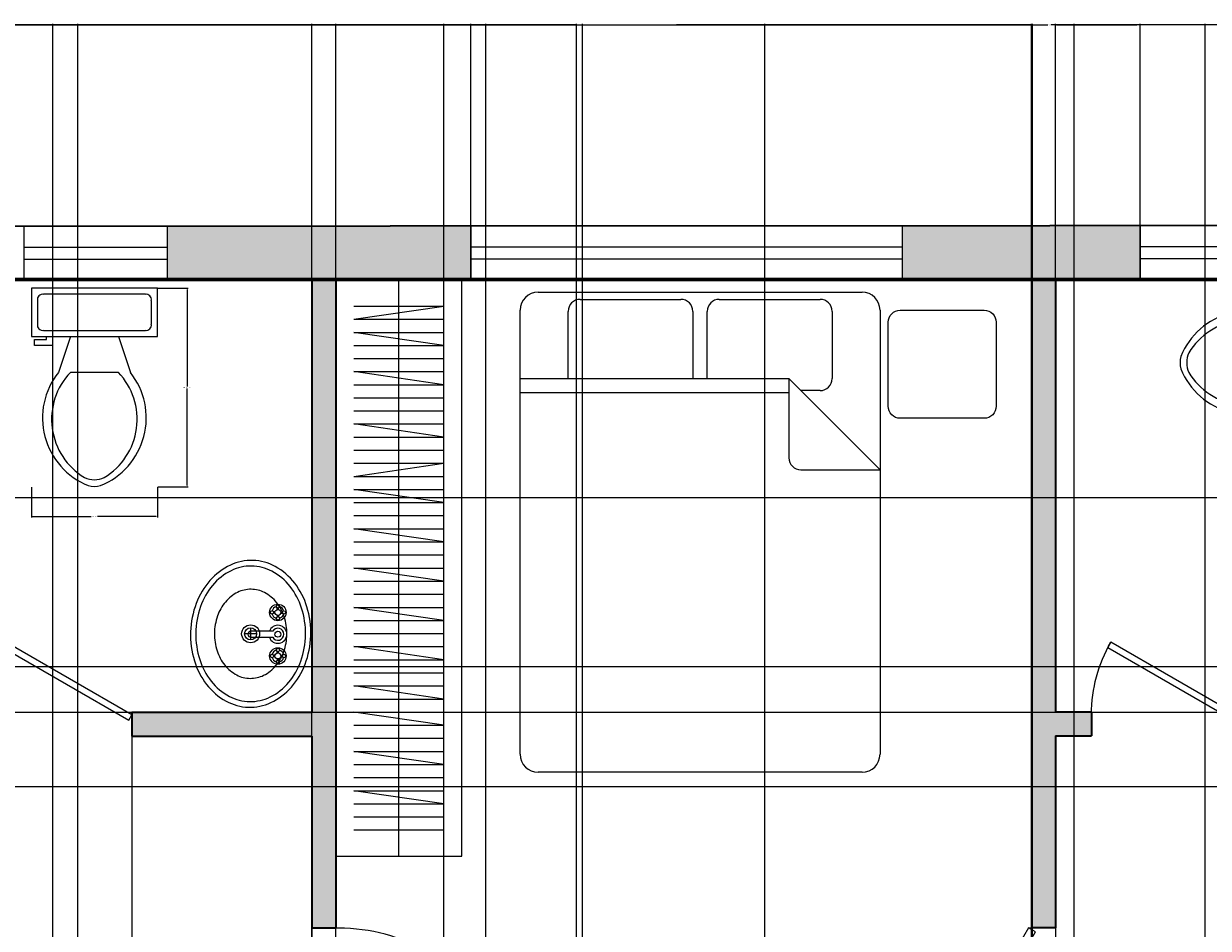
# Model space of a CAD drawing. Units: inches. Extents: x 1531 to 2263, y 2711 to 3216.
# Tile 6 of 12: x 1728 to 1925, y 3066 to 3216. Entities that reach past the tile are written whole.
import ezdxf

# ---------------------------------------------------------------- set-up
doc = ezdxf.new("R2010")
doc.units = ezdxf.units.IN
for name, color, linetype, lineweight in [('A-ANNO-DIMS', 2, 'Continuous', 18), ('A-DOOR', 3, 'Continuous', 25), ('A-FLOR-CASE', 9, 'Continuous', 18), ('A-FLOR-FIXT', 9, 'Continuous', 18), ('A-FURN', 8, 'Continuous', 18), ('A-GLAZ', 4, 'Continuous', 18), ('A-WALL', 7, 'Continuous', 35)]:
    doc.layers.add(name, color=color, linetype=linetype, lineweight=lineweight)
doc.layers.add('A-WALL-PATT', color=18, linetype='Continuous', lineweight=13, true_color=0x000000)
doc.styles.get("Standard").update_dxf_attribs({"font": 'arial.ttf'})
doc.dimstyles.get("Standard").update_dxf_attribs({"dimtxt": 0.18, "dimasz": 0.18, "dimexe": 0.18, "dimexo": 0.0625, "dimgap": 0.09, "dimtad": 0, "dimtih": 1, "dimtoh": 1, "dimdec": 4, "dimzin": 0, "dimdsep": 46, "dimtxsty": 'Standard', "dimcen": 0.09, "dimadec": 0, "dimazin": 0, "dimtfac": 1, "dimtdec": 4, "dimtofl": 0, "dimtmove": 0, "dimatfit": 3, "dimfxl": 1, "dimtolj": 1, "dimtzin": 0, "dimarcsym": 0})

# ---------------------------------------------------------------- blocks, each defined once
blk = doc.blocks.new('*U3')
for p, q in [((0, 0), (0, -6)), ((40, 0), (40, -6))]:
    blk.add_line(p, q)
blk.add_lwpolyline([(0, 0), (34.64, 20), (35.52, 18.48), (0.87, -1.52)], close=True)
blk.add_arc((0, 0), 40, 0, 30)
blk = doc.blocks.new('*U5')
for p, q in [((0, 0), (0, -6)), ((-40, 0), (-40, -6))]:
    blk.add_line(p, q)
blk.add_lwpolyline([(0, 0), (-34.64, 20), (-35.52, 18.48), (-0.88, -1.52)], close=True)
blk.add_arc((0, 0), 40, 150, 180)
blk = doc.blocks.new('*U6')
for p, q in [((0, 0), (0, 6)), ((40, 0), (40, 6))]:
    blk.add_line(p, q)
blk.add_lwpolyline([(0, 0), (34.64, -20), (35.52, -18.48), (0.87, 1.52)], close=True)
blk.add_arc((0, 0), 40, 330, 0)
blk = doc.blocks.new('Toilet - top')
for p, q in [((9.5, -6), (9.5, -2)), ((-10, -8.5), (-8, -8.5)), ((-10, -9.5), (-10, -8.5)), ((-7, -9.5), (-10, -9.5)), ((-8, -8.5), (-8, -8)), ((-7, -8), (-7, -9.5)), ((-4, -8), (-6, -14)), ((4, -8), (6, -14)), ((4, -14), (-4, -14))]:
    blk.add_line(p, q)
blk.add_lwpolyline([(10.5, -8), (10.5, 0), (-10.5, 0), (-10.5, -8)], close=True)
for points in [[(8.5, -1), (-8.5, -1)], [(-9.5, -2), (-9.5, -6)], [(-8.5, -7), (8.5, -7)]]:
    blk.add_lwpolyline(points)
for centre, radius, start, end in [((-8.62, -1.88), 0.884, 81.8699, 188.1301), ((8.62, -1.88), 0.884, 351.8699, 98.1301), ((-8.62, -6.12), 0.884, 171.8699, 278.1301), ((8.62, -6.12), 0.884, 261.8699, 8.1301), ((3.52, -21.58), 12.17, 141.4691, 247.9714), ((4.2, -21.82), 11.33, 136.3677, 238.9468), ((-3.52, -21.58), 12.17, 292.0284, 38.5307), ((-4.2, -21.82), 11.33, 301.053, 43.6321), ((0, -27.88), 4, 245.7318, 294.2682), ((0, -29), 4, 254.8605, 285.1395)]:
    blk.add_arc(centre, radius, start, end)
blk = doc.blocks.new('Bed - Queen')
for p, q in [((3, 0), (57, 0)), ((10, -1.2), (26.8, -1.2)), ((33.2, -1.2), (50, -1.2)), ((0, -77), (0, -3)), ((8, -14.4), (8, -3.2)), ((28.8, -3.2), (28.8, -14.4)), ((31.2, -14.4), (31.2, -3.2)), ((52, -3.2), (52, -14.4)), ((60, -3), (60, -77)), ((0, -14.4), (44.8, -14.4)), ((60, -29.6), (44.8, -14.4)), ((44.8, -14.4), (44.8, -27.6)), ((44.8, -16.8), (0, -16.8)), ((50, -16.4), (46.8, -16.4)), ((46.8, -29.6), (60, -29.6)), ((57, -80), (3, -80))]:
    blk.add_line(p, q)
blk.add_lwpolyline([(63.37, -3.02), (77.37, -3.02, -0.414214), (79.37, -5.02), (79.37, -19.02, -0.414214), (77.37, -21.02), (63.37, -21.02, -0.414214), (61.37, -19.02), (61.37, -5.02, -0.414214)], format="xyb", close=True)
for centre, radius, start, end in [((3, -3), 3, 90, 180), ((57, -3), 3, 0, 90), ((10, -3.2), 2, 90, 180), ((26.8, -3.2), 2, 0, 90), ((33.2, -3.2), 2, 90, 180), ((50, -3.2), 2, 0, 90), ((50, -14.4), 2, 270, 0), ((46.8, -27.6), 2, 180, 270), ((3, -77), 3, 180, 270), ((57, -77), 3, 270, 0)]:
    blk.add_arc(centre, radius, start, end)
blk = doc.blocks.new('Sink - Oval top')
for p, q in [((-1, 0), (1, 0)), ((0, 1), (0, -1))]:
    blk.add_line(p, q)
for points in [[(-12.23, 0.39, 0.117634), (-11.46, -3.36, 0.104469), (-8.88, -6.8, 0.090016), (-5.08, -9.07, 0.08192), (-0.32, -10.02, 0.08192), (4.49, -9.38, 0.090016), (8.42, -7.36, 0.104469), (11.22, -4.09, 0.117634), (12.23, -0.39, 0.117634), (11.46, 3.36, 0.104469), (8.88, 6.8, 0.090016), (5.08, 9.07, 0.08192), (0.32, 10.02, 0.08192), (-4.49, 9.38, 0.090016), (-8.42, 7.36, 0.104469), (-11.22, 4.09, 0.117634)], [(-11.29, 0.16, 0.118622), (-10.52, -3.25, 0.104678), (-8.07, -6.36, 0.089562), (-4.54, -8.37, 0.081185), (-0.13, -9.15, 0.081185), (4.3, -8.49, 0.089562), (7.89, -6.58, 0.104678), (10.42, -3.55, 0.118622), (11.29, -0.16, 0.118622), (10.52, 3.25, 0.104678), (8.07, 6.36, 0.089562), (4.54, 8.37, 0.081185), (0.13, 9.15, 0.081185), (-4.3, 8.49, 0.089562), (-7.89, 6.58, 0.104678), (-10.42, 3.55, 0.118622)], [(-7.42, 0.08, 0.118283), (-6.91, -2.17, 0.104607), (-5.29, -4.21, 0.089718), (-2.97, -5.53, 0.081436), (-0.07, -6.04, 0.081436), (2.84, -5.59, 0.089718), (5.2, -4.33, 0.104607), (6.86, -2.32, 0.118283), (7.42, -0.08, 0.118283), (6.91, 2.17, 0.104607), (5.29, 4.21, 0.089718), (2.97, 5.53, 0.081436), (0.07, 6.04, 0.081436), (-2.84, 5.59, 0.089718), (-5.2, 4.33, 0.104607), (-6.86, 2.32, 0.118283)]]:
    blk.add_lwpolyline(points, format="xyb", close=True)
for radius in [1.5, 1]:
    blk.add_circle((0, 0), radius)
blk = doc.blocks.new('Faucet - Bathroom top')
for p, q in [((-4.107, 0.125), (-4.375, 0.125)), ((-3.75, 0.4788), (-3.75, 0.75)), ((-3.5, 0.482), (-3.5, 0.75)), ((-3.1461, 0.125), (-2.875, 0.125)), ((3.143, 0.125), (2.875, 0.125)), ((3.5, 0.4788), (3.5, 0.75)), ((3.75, 0.482), (3.75, 0.75)), ((4.1039, 0.125), (4.375, 0.125)), ((-4.1039, -0.125), (-4.375, -0.125)), ((-3.75, -0.4821), (-3.75, -0.75)), ((-3.5, -0.4789), (-3.5, -0.75)), ((-3.143, -0.125), (-2.875, -0.125)), ((-0.5, -0.8639), (-0.5, -4.5)), ((0.5, -4.5), (0.5, -0.8631)), ((3.1461, -0.125), (2.875, -0.125)), ((3.5, -0.4821), (3.5, -0.75)), ((3.75, -0.4789), (3.75, -0.75)), ((4.107, -0.125), (4.375, -0.125))]:
    blk.add_line(p, q)
for centre, radius in [((-3.625, 0), 1.375), ((-4.625, 0), 0.2795), ((-3.625, 0), 0.5), ((-3.625, 1), 0.2795), ((-2.625, 0), 0.2795), ((0, 0), 0.5), ((3.625, 0), 1.375), ((2.625, 0), 0.2795), ((3.625, 0), 0.5), ((3.625, 1), 0.2795), ((4.625, 0), 0.2795), ((-3.625, -1), 0.2795), ((3.625, -1), 0.2795)]:
    blk.add_circle(centre, radius)
for centre, radius, start, end in [((-3.625, 0), 1, 105.2407, 164.2093), ((-3.625, 0), 1, 16.44125, 74.07887), ((0, 0), 1.5, 289.6514, 250.3603), ((0, 0), 1, 300.3431, 239.7554), ((3.625, 0), 1, 106.12, 164.0884), ((3.625, 0), 1, 16.23422, 73.90469), ((-3.625, 0), 1, 196.2342, 253.9047), ((-3.625, 0), 1, 286.12, 344.0884), ((3.625, 0), 1, 196.4413, 254.0789), ((3.625, 0), 1, 285.2407, 344.2093), ((0, -4.5), 0.5, 180, 0)]:
    blk.add_arc(centre, radius, start, end)
blk = doc.blocks.new('WIN-72IN')
for p, q in [((0, 5.5), (72, 5.5)), ((0, 3.5), (72, 3.5))]:
    blk.add_line(p, q)
for points in [[(0, 9), (0, 0)], [(72, 0), (72, 9)]]:
    blk.add_lwpolyline(points)
blk = doc.blocks.new('WIN-24IN')
for p, q in [((0, 5.5), (24, 5.5)), ((0, 3.5), (24, 3.5))]:
    blk.add_line(p, q)
for points in [[(0, 9), (0, 0)], [(24, 0), (24, 9)]]:
    blk.add_lwpolyline(points)
blk = doc.blocks.new('WARDROBE-96IN')
for p, q in [((96, 21), (0, 21)), ((0, 21), (0, 0)), ((0, 0), (0, 21)), ((96, 0), (96, 21)), ((4.36, 3), (4.36, 18)), ((6.55, 3), (4.36, 18)), ((6.55, 3), (6.55, 18)), ((8.73, 3), (8.73, 18)), ((10.91, 18), (8.73, 3)), ((10.91, 3), (10.91, 18)), ((13.09, 3), (13.09, 18)), ((15.27, 3), (15.27, 18)), ((17.45, 18), (15.27, 3)), ((17.45, 3), (17.45, 18)), ((19.64, 3), (19.64, 18)), ((21.82, 3), (21.82, 18)), ((24, 3), (24, 18)), ((26.18, 18), (24, 3)), ((26.18, 3), (26.18, 18)), ((28.36, 3), (28.36, 18)), ((30.55, 3), (30.55, 18)), ((32.73, 3), (30.55, 18)), ((32.73, 3), (32.73, 18)), ((34.91, 3), (34.91, 18)), ((37.09, 18), (34.91, 3)), ((37.09, 3), (37.09, 18)), ((39.27, 3), (39.27, 18)), ((41.45, 3), (41.45, 18)), ((43.64, 18), (41.45, 3)), ((43.64, 3), (43.64, 18)), ((45.82, 3), (45.82, 18)), ((48, 3), (48, 18)), ((50.18, 18), (48, 3)), ((50.18, 3), (50.18, 18)), ((52.36, 3), (52.36, 18)), ((54.55, 3), (54.55, 18)), ((56.73, 18), (54.55, 3)), ((56.73, 3), (56.73, 18)), ((58.91, 3), (58.91, 18)), ((61.09, 3), (61.09, 18)), ((63.27, 18), (61.09, 3)), ((63.27, 3), (63.27, 18)), ((65.45, 3), (65.45, 18)), ((67.64, 3), (67.64, 18)), ((69.82, 18), (67.64, 3)), ((69.82, 3), (69.82, 18)), ((72, 3), (72, 18)), ((74.18, 18), (72, 3)), ((74.18, 3), (74.18, 18)), ((76.36, 3), (76.36, 18)), ((78.55, 3), (78.55, 18)), ((80.73, 18), (78.55, 3)), ((80.73, 3), (80.73, 18)), ((82.91, 3), (82.91, 18)), ((85.09, 3), (85.09, 18)), ((87.27, 18), (85.09, 3)), ((87.27, 3), (87.27, 18)), ((89.45, 3), (89.45, 18)), ((91.64, 3), (91.64, 18)), ((96, 10.5), (0, 10.5)), ((0, 0), (96, 0))]:
    blk.add_line(p, q)
blk = doc.blocks.new('*D36')
at = {"layer": 'A-ANNO-DIMS', "color": 0, "lineweight": -2, "transparency": 16777216}
for p, q in [((1750.21, 3172.39), (1755.29, 3172.39)), ((1755.11, 3172.21), (1755.11, 3156.05)), ((1755.11, 3139.52), (1755.11, 3155.68)), ((1750.21, 3139.34), (1755.29, 3139.34))]:
    blk.add_line(p, q, dxfattribs=at)
at = {"layer": 'A-ANNO-DIMS', "color": 0, "transparency": 16777216}
for points in [[(1755.08, 3172.21), (1755.14, 3172.21), (1755.11, 3172.39)], [(1755.08, 3139.52), (1755.14, 3139.52), (1755.11, 3139.34)]]:
    blk.add_solid(points, dxfattribs=at)
at = {"layer": 'Defpoints', "color": 0, "transparency": 16777216}
for p in [(1750.15, 3172.39), (1755.11, 3172.39), (1750.15, 3139.34)]:
    blk.add_point(p, dxfattribs=at)
at = {"layer": 'A-ANNO-DIMS', "color": 0, "transparency": 16777216, "insert": (1755.11, 3155.86), "char_height": 0.18, "attachment_point": 5}
blk.add_mtext('\\A1;WC 33 TYP.', dxfattribs=at)
blk = doc.blocks.new('*D37')
at = {"layer": 'A-ANNO-DIMS', "color": 0, "lineweight": -2, "transparency": 16777216}
for p, q in [((1729.15, 3139.28), (1729.15, 3134.2)), ((1750.15, 3139.28), (1750.15, 3134.2)), ((1729.33, 3134.38), (1739.12, 3134.38)), ((1749.97, 3134.38), (1740.18, 3134.38))]:
    blk.add_line(p, q, dxfattribs=at)
at = {"layer": 'A-ANNO-DIMS', "color": 0, "transparency": 16777216}
for points in [[(1729.33, 3134.41), (1729.33, 3134.35), (1729.15, 3134.38)], [(1749.97, 3134.41), (1749.97, 3134.35), (1750.15, 3134.38)]]:
    blk.add_solid(points, dxfattribs=at)
at = {"layer": 'Defpoints', "color": 0, "transparency": 16777216}
for p in [(1729.15, 3139.34), (1750.15, 3139.34), (1750.15, 3134.38)]:
    blk.add_point(p, dxfattribs=at)
at = {"layer": 'A-ANNO-DIMS', "color": 0, "transparency": 16777216, "insert": (1739.65, 3134.38), "char_height": 0.18, "attachment_point": 5}
blk.add_mtext('\\A1;21 TYP.', dxfattribs=at)
blk = doc.blocks.new('*D54')
at = {"layer": 'A-ANNO-DIMS', "color": 0, "lineweight": -2, "transparency": 16777216}
for p, q in [((1568.91, 3182.74), (1568.91, 3216.47)), ((1569.09, 3216.29), (1898.62, 3216.29)), ((2228.73, 3216.29), (1899.2, 3216.29)), ((2228.91, 3183.08), (2228.91, 3216.47))]:
    blk.add_line(p, q, dxfattribs=at)
at = {"layer": 'A-ANNO-DIMS', "color": 0, "transparency": 16777216}
for points in [[(1569.09, 3216.32), (1569.09, 3216.26), (1568.91, 3216.29)], [(2228.73, 3216.32), (2228.73, 3216.26), (2228.91, 3216.29)]]:
    blk.add_solid(points, dxfattribs=at)
at = {"layer": 'Defpoints', "color": 0, "transparency": 16777216}
for p in [(2228.91, 3216.29), (1568.91, 3182.67), (2228.91, 3183.02)]:
    blk.add_point(p, dxfattribs=at)
at = {"layer": 'A-ANNO-DIMS', "color": 0, "transparency": 16777216, "insert": (1898.91, 3216.29), "char_height": 0.18, "attachment_point": 5}
blk.add_mtext('\\A1;660', dxfattribs=at)
blk = doc.blocks.new('*D58')
at = {"layer": 'A-ANNO-DIMS', "color": 0, "lineweight": -2, "transparency": 16777216}
for p, q in [((1715.91, 3097.69), (1715.91, 2711.06)), ((1775.91, 3097.72), (1775.91, 2711.06)), ((1716.09, 2711.24), (1745.69, 2711.24)), ((1775.73, 2711.24), (1746.13, 2711.24))]:
    blk.add_line(p, q, dxfattribs=at)
at = {"layer": 'A-ANNO-DIMS', "color": 0, "transparency": 16777216}
for points in [[(1716.09, 2711.27), (1716.09, 2711.21), (1715.91, 2711.24)], [(1775.73, 2711.27), (1775.73, 2711.21), (1775.91, 2711.24)]]:
    blk.add_solid(points, dxfattribs=at)
at = {"layer": 'Defpoints', "color": 0, "transparency": 16777216}
for p in [(1715.91, 3097.75), (1775.91, 3097.78), (1775.91, 2711.24)]:
    blk.add_point(p, dxfattribs=at)
at = {"layer": 'A-ANNO-DIMS', "color": 0, "transparency": 16777216, "insert": (1745.91, 2711.24), "char_height": 0.18, "attachment_point": 5}
blk.add_mtext('\\A1;60', dxfattribs=at)
blk = doc.blocks.new('*D59')
at = {"layer": 'A-ANNO-DIMS', "color": 0, "lineweight": -2, "transparency": 16777216}
for p, q in [((1779.91, 3029.85), (1779.91, 3216.47)), ((1780.09, 3216.29), (1837.63, 3216.29)), ((1895.73, 3216.29), (1838.19, 3216.29)), ((1895.91, 3029.91), (1895.91, 3216.47))]:
    blk.add_line(p, q, dxfattribs=at)
at = {"layer": 'A-ANNO-DIMS', "color": 0, "transparency": 16777216}
for points in [[(1780.09, 3216.32), (1780.09, 3216.26), (1779.91, 3216.29)], [(1895.73, 3216.32), (1895.73, 3216.26), (1895.91, 3216.29)]]:
    blk.add_solid(points, dxfattribs=at)
at = {"layer": 'Defpoints', "color": 0, "transparency": 16777216}
for p in [(1895.91, 3216.29), (1895.91, 3029.85), (1779.91, 3029.79)]:
    blk.add_point(p, dxfattribs=at)
at = {"layer": 'A-ANNO-DIMS', "color": 0, "transparency": 16777216, "insert": (1837.91, 3216.29), "char_height": 0.18, "attachment_point": 5}
blk.add_mtext('\\A1;116', dxfattribs=at)
blk = doc.blocks.new('*D60')
at = {"layer": 'A-ANNO-DIMS', "color": 0, "lineweight": -2, "transparency": 16777216}
for p, q in [((1899.91, 3097.79), (1899.91, 2711.06)), ((1955.91, 3097.81), (1955.91, 2711.06)), ((1900.09, 2711.24), (1927.69, 2711.24)), ((1955.73, 2711.24), (1928.13, 2711.24))]:
    blk.add_line(p, q, dxfattribs=at)
at = {"layer": 'A-ANNO-DIMS', "color": 0, "transparency": 16777216}
for points in [[(1900.09, 2711.27), (1900.09, 2711.21), (1899.91, 2711.24)], [(1955.73, 2711.27), (1955.73, 2711.21), (1955.91, 2711.24)]]:
    blk.add_solid(points, dxfattribs=at)
at = {"layer": 'Defpoints', "color": 0, "transparency": 16777216}
for p in [(1899.91, 3097.85), (1955.91, 3097.88), (1955.91, 2711.24)]:
    blk.add_point(p, dxfattribs=at)
at = {"layer": 'A-ANNO-DIMS', "color": 0, "transparency": 16777216, "insert": (1927.91, 2711.24), "char_height": 0.18, "attachment_point": 5}
blk.add_mtext('\\A1;56', dxfattribs=at)
blk = doc.blocks.new('*D66')
at = {"layer": 'A-ANNO-DIMS', "color": 0, "lineweight": -2, "transparency": 16777216}
for p, q in [((1577.91, 2895.74), (1577.91, 3216.47)), ((1578.09, 3216.29), (1676.63, 3216.29)), ((1775.73, 3216.29), (1677.19, 3216.29)), ((1775.91, 2895.85), (1775.91, 3216.47))]:
    blk.add_line(p, q, dxfattribs=at)
at = {"layer": 'A-ANNO-DIMS', "color": 0, "transparency": 16777216}
for points in [[(1578.09, 3216.32), (1578.09, 3216.26), (1577.91, 3216.29)], [(1775.73, 3216.32), (1775.73, 3216.26), (1775.91, 3216.29)]]:
    blk.add_solid(points, dxfattribs=at)
at = {"layer": 'Defpoints', "color": 0, "transparency": 16777216}
for p in [(1775.91, 3216.29), (1577.91, 2895.68), (1775.91, 2895.78)]:
    blk.add_point(p, dxfattribs=at)
at = {"layer": 'A-ANNO-DIMS', "color": 0, "transparency": 16777216, "insert": (1676.91, 3216.29), "char_height": 0.18, "attachment_point": 5}
blk.add_mtext('\\A1;198', dxfattribs=at)
blk = doc.blocks.new('*D68')
at = {"layer": 'A-ANNO-DIMS', "color": 0, "lineweight": -2, "transparency": 16777216}
for p, q in [((1736.91, 2839.83), (1736.91, 3216.47)), ((1737.09, 3216.29), (1770.69, 3216.29)), ((1804.73, 3216.29), (1771.13, 3216.29)), ((1804.91, 2839.86), (1804.91, 3216.47))]:
    blk.add_line(p, q, dxfattribs=at)
at = {"layer": 'A-ANNO-DIMS', "color": 0, "transparency": 16777216}
for points in [[(1737.09, 3216.32), (1737.09, 3216.26), (1736.91, 3216.29)], [(1804.73, 3216.32), (1804.73, 3216.26), (1804.91, 3216.29)]]:
    blk.add_solid(points, dxfattribs=at)
at = {"layer": 'Defpoints', "color": 0, "transparency": 16777216}
for p in [(1804.91, 3216.29), (1736.91, 2839.76), (1804.91, 2839.8)]:
    blk.add_point(p, dxfattribs=at)
at = {"layer": 'A-ANNO-DIMS', "color": 0, "transparency": 16777216, "insert": (1770.91, 3216.29), "char_height": 0.18, "attachment_point": 5}
blk.add_mtext('\\A1;68', dxfattribs=at)
blk = doc.blocks.new('*D80')
at = {"layer": 'A-ANNO-DIMS', "color": 0, "lineweight": -2, "transparency": 16777216}
for p, q in [((1715.97, 3173.75), (2262.37, 3173.75)), ((2262.19, 3173.57), (2262.19, 3137.93)), ((2262.19, 3101.93), (2262.19, 3137.57)), ((1715.97, 3101.75), (2262.37, 3101.75))]:
    blk.add_line(p, q, dxfattribs=at)
at = {"layer": 'A-ANNO-DIMS', "color": 0, "transparency": 16777216}
for points in [[(2262.16, 3173.57), (2262.22, 3173.57), (2262.19, 3173.75)], [(2262.16, 3101.93), (2262.22, 3101.93), (2262.19, 3101.75)]]:
    blk.add_solid(points, dxfattribs=at)
at = {"layer": 'Defpoints', "color": 0, "transparency": 16777216}
for p in [(1715.91, 3173.75), (1715.91, 3101.75), (2262.19, 3101.75)]:
    blk.add_point(p, dxfattribs=at)
at = {"layer": 'A-ANNO-DIMS', "color": 0, "transparency": 16777216, "insert": (2262.19, 3137.75), "char_height": 0.18, "attachment_point": 5}
blk.add_mtext('\\A1;72', dxfattribs=at)
blk = doc.blocks.new('*D85')
at = {"layer": 'A-ANNO-DIMS', "color": 0, "lineweight": -2, "transparency": 16777216}
for p, q in [((2079.85, 3173.94), (1531.04, 3173.94)), ((1531.22, 3173.76), (1531.22, 3131.82)), ((1531.22, 3089.52), (1531.22, 3131.46)), ((2079.85, 3089.34), (1531.04, 3089.34))]:
    blk.add_line(p, q, dxfattribs=at)
at = {"layer": 'A-ANNO-DIMS', "color": 0, "transparency": 16777216}
for points in [[(1531.19, 3173.76), (1531.25, 3173.76), (1531.22, 3173.94)], [(1531.19, 3089.52), (1531.25, 3089.52), (1531.22, 3089.34)]]:
    blk.add_solid(points, dxfattribs=at)
at = {"layer": 'Defpoints', "color": 0, "transparency": 16777216}
for p in [(1531.22, 3173.94), (2079.91, 3173.94), (2079.91, 3089.34)]:
    blk.add_point(p, dxfattribs=at)
at = {"layer": 'A-ANNO-DIMS', "color": 0, "transparency": 16777216, "insert": (1531.22, 3131.64), "char_height": 0.18, "attachment_point": 5}
blk.add_mtext('\\A1;84.6', dxfattribs=at)
blk = doc.blocks.new('*D87')
at = {"layer": 'A-ANNO-DIMS', "color": 0, "lineweight": -2, "transparency": 16777216}
for p, q in [((1721.91, 3101.69), (1721.91, 2711.06)), ((1745.91, 3101.7), (1745.91, 2711.06)), ((1722.09, 2711.24), (1733.69, 2711.24)), ((1745.73, 2711.24), (1734.13, 2711.24))]:
    blk.add_line(p, q, dxfattribs=at)
at = {"layer": 'A-ANNO-DIMS', "color": 0, "transparency": 16777216}
for points in [[(1722.09, 2711.27), (1722.09, 2711.21), (1721.91, 2711.24)], [(1745.73, 2711.27), (1745.73, 2711.21), (1745.91, 2711.24)]]:
    blk.add_solid(points, dxfattribs=at)
at = {"layer": 'Defpoints', "color": 0, "transparency": 16777216}
for p in [(1721.91, 3101.75), (1745.91, 3101.77), (1745.91, 2711.24)]:
    blk.add_point(p, dxfattribs=at)
at = {"layer": 'A-ANNO-DIMS', "color": 0, "transparency": 16777216, "insert": (1733.91, 2711.24), "char_height": 0.18, "attachment_point": 5}
blk.add_mtext('\\A1;24', dxfattribs=at)
blk = doc.blocks.new('*D90')
at = {"layer": 'A-ANNO-DIMS', "color": 0, "lineweight": -2, "transparency": 16777216}
for p, q in [((1779.91, 3173.85), (1779.91, 3216.47)), ((1780.09, 3216.29), (1790.76, 3216.29)), ((1802.21, 3216.29), (1791.55, 3216.29)), ((1802.39, 3173.86), (1802.39, 3216.47))]:
    blk.add_line(p, q, dxfattribs=at)
at = {"layer": 'A-ANNO-DIMS', "color": 0, "transparency": 16777216}
for points in [[(1780.09, 3216.32), (1780.09, 3216.26), (1779.91, 3216.29)], [(1802.21, 3216.32), (1802.21, 3216.26), (1802.39, 3216.29)]]:
    blk.add_solid(points, dxfattribs=at)
at = {"layer": 'Defpoints', "color": 0, "transparency": 16777216}
for p in [(1802.39, 3216.29), (1779.91, 3173.79), (1802.39, 3173.8)]:
    blk.add_point(p, dxfattribs=at)
at = {"layer": 'A-ANNO-DIMS', "color": 0, "transparency": 16777216, "insert": (1791.15, 3216.29), "char_height": 0.18, "attachment_point": 5}
blk.add_mtext('\\A1;22.48', dxfattribs=at)
blk = doc.blocks.new('*D91')
at = {"layer": 'A-ANNO-DIMS', "color": 0, "lineweight": -2, "transparency": 16777216}
for p, q in [((1899.91, 3173.91), (1899.91, 3216.47)), ((1900.09, 3216.29), (1906.51, 3216.29)), ((1913.84, 3216.29), (1907.42, 3216.29)), ((1914.02, 3173.92), (1914.02, 3216.47))]:
    blk.add_line(p, q, dxfattribs=at)
at = {"layer": 'A-ANNO-DIMS', "color": 0, "transparency": 16777216}
for points in [[(1900.09, 3216.32), (1900.09, 3216.26), (1899.91, 3216.29)], [(1913.84, 3216.32), (1913.84, 3216.26), (1914.02, 3216.29)]]:
    blk.add_solid(points, dxfattribs=at)
at = {"layer": 'Defpoints', "color": 0, "transparency": 16777216}
for p in [(1914.02, 3216.29), (1899.91, 3173.85), (1914.02, 3173.86)]:
    blk.add_point(p, dxfattribs=at)
at = {"layer": 'A-ANNO-DIMS', "color": 0, "transparency": 16777216, "insert": (1906.97, 3216.29), "char_height": 0.18, "attachment_point": 5}
blk.add_mtext('\\A1;14.113', dxfattribs=at)
blk = doc.blocks.new('*D98')
at = {"layer": 'A-ANNO-DIMS', "color": 0, "lineweight": -2, "transparency": 16777216}
for p, q in [((1820.04, 3001.95), (1820.04, 3216.47)), ((1820.22, 3216.29), (1857.83, 3216.29)), ((1895.86, 3216.29), (1858.26, 3216.29)), ((1896.04, 3001.95), (1896.04, 3216.47))]:
    blk.add_line(p, q, dxfattribs=at)
at = {"layer": 'A-ANNO-DIMS', "color": 0, "transparency": 16777216}
for points in [[(1820.22, 3216.32), (1820.22, 3216.26), (1820.04, 3216.29)], [(1895.86, 3216.32), (1895.86, 3216.26), (1896.04, 3216.29)]]:
    blk.add_solid(points, dxfattribs=at)
at = {"layer": 'Defpoints', "color": 0, "transparency": 16777216}
for p in [(1896.04, 3216.29), (1820.04, 3001.89), (1896.04, 3001.89)]:
    blk.add_point(p, dxfattribs=at)
at = {"layer": 'A-ANNO-DIMS', "color": 0, "transparency": 16777216, "insert": (1858.04, 3216.29), "char_height": 0.18, "attachment_point": 5}
blk.add_mtext('\\A1;76', dxfattribs=at)
blk = doc.blocks.new('*D100')
at = {"layer": 'A-ANNO-DIMS', "color": 0, "lineweight": -2, "transparency": 16777216}
for p, q in [((2219.85, 3174.02), (1531.04, 3174.02)), ((1531.22, 3173.84), (1531.22, 3155.93)), ((1531.22, 3137.67), (1531.22, 3155.57)), ((2219.85, 3137.49), (1531.04, 3137.49))]:
    blk.add_line(p, q, dxfattribs=at)
at = {"layer": 'A-ANNO-DIMS', "color": 0, "transparency": 16777216}
for points in [[(1531.19, 3173.84), (1531.25, 3173.84), (1531.22, 3174.02)], [(1531.19, 3137.67), (1531.25, 3137.67), (1531.22, 3137.49)]]:
    blk.add_solid(points, dxfattribs=at)
at = {"layer": 'Defpoints', "color": 0, "transparency": 16777216}
for p in [(2219.91, 3174.02), (1531.22, 3137.49), (2219.91, 3137.49)]:
    blk.add_point(p, dxfattribs=at)
at = {"layer": 'A-ANNO-DIMS', "color": 0, "transparency": 16777216, "insert": (1531.22, 3155.75), "char_height": 0.18, "attachment_point": 5}
blk.add_mtext('\\A1;36.526', dxfattribs=at)
blk = doc.blocks.new('*D103')
at = {"layer": 'A-ANNO-DIMS', "color": 0, "lineweight": -2, "transparency": 16777216}
for p, q in [((1577.97, 3173.68), (2262.37, 3173.68)), ((2262.19, 3173.5), (2262.19, 3141.71)), ((2262.19, 3109.55), (2262.19, 3141.34)), ((1577.97, 3109.37), (2262.37, 3109.37))]:
    blk.add_line(p, q, dxfattribs=at)
at = {"layer": 'A-ANNO-DIMS', "color": 0, "transparency": 16777216}
for points in [[(2262.16, 3173.5), (2262.22, 3173.5), (2262.19, 3173.68)], [(2262.16, 3109.55), (2262.22, 3109.55), (2262.19, 3109.37)]]:
    blk.add_solid(points, dxfattribs=at)
at = {"layer": 'Defpoints', "color": 0, "transparency": 16777216}
for p in [(1577.91, 3173.68), (1577.91, 3109.37), (2262.19, 3109.37)]:
    blk.add_point(p, dxfattribs=at)
at = {"layer": 'A-ANNO-DIMS', "color": 0, "transparency": 16777216, "insert": (2262.19, 3141.52), "char_height": 0.18, "attachment_point": 5}
blk.add_mtext('\\A1;64.31', dxfattribs=at)
blk = doc.blocks.new('*D115')
at = {"layer": 'A-ANNO-DIMS', "color": 0, "lineweight": -2, "transparency": 16777216}
for p, q in [((1779.91, 2993.83), (1779.91, 3216.47)), ((1780.09, 3216.29), (1799.58, 3216.29)), ((1819.86, 3216.29), (1800.37, 3216.29)), ((1820.04, 3001.95), (1820.04, 3216.47))]:
    blk.add_line(p, q, dxfattribs=at)
at = {"layer": 'A-ANNO-DIMS', "color": 0, "transparency": 16777216}
for points in [[(1780.09, 3216.32), (1780.09, 3216.26), (1779.91, 3216.29)], [(1819.86, 3216.32), (1819.86, 3216.26), (1820.04, 3216.29)]]:
    blk.add_solid(points, dxfattribs=at)
at = {"layer": 'Defpoints', "color": 0, "transparency": 16777216}
for p in [(1820.04, 3216.29), (1820.04, 3001.89), (1779.91, 2993.76)]:
    blk.add_point(p, dxfattribs=at)
at = {"layer": 'A-ANNO-DIMS', "color": 0, "transparency": 16777216, "insert": (1799.98, 3216.29), "char_height": 0.18, "attachment_point": 5}
blk.add_mtext('\\A1;40.13', dxfattribs=at)
blk = doc.blocks.new('*D117')
at = {"layer": 'A-ANNO-DIMS', "color": 0, "lineweight": -2, "transparency": 16777216}
for p, q in [((1821.02, 2965.7), (1821.02, 3216.47)), ((1821.2, 3216.29), (1835.77, 3216.29)), ((1851.26, 3216.29), (1836.69, 3216.29)), ((1851.44, 2965.7), (1851.44, 3216.47))]:
    blk.add_line(p, q, dxfattribs=at)
at = {"layer": 'A-ANNO-DIMS', "color": 0, "transparency": 16777216}
for points in [[(1821.2, 3216.32), (1821.2, 3216.26), (1821.02, 3216.29)], [(1851.26, 3216.32), (1851.26, 3216.26), (1851.44, 3216.29)]]:
    blk.add_solid(points, dxfattribs=at)
at = {"layer": 'Defpoints', "color": 0, "transparency": 16777216}
for p in [(1851.44, 3216.29), (1821.02, 2965.63), (1851.44, 2965.63)]:
    blk.add_point(p, dxfattribs=at)
at = {"layer": 'A-ANNO-DIMS', "color": 0, "transparency": 16777216, "insert": (1836.23, 3216.29), "char_height": 0.18, "attachment_point": 5}
blk.add_mtext('\\A1;30.417', dxfattribs=at)
blk = doc.blocks.new('*D119')
at = {"layer": 'A-ANNO-DIMS', "color": 0, "lineweight": -2, "transparency": 16777216}
for p, q in [((1779.91, 2993.83), (1779.91, 3216.47)), ((1780.09, 3216.29), (1788.7, 3216.29)), ((1797.73, 3216.29), (1789.12, 3216.29)), ((1797.91, 2993.83), (1797.91, 3216.47))]:
    blk.add_line(p, q, dxfattribs=at)
at = {"layer": 'A-ANNO-DIMS', "color": 0, "transparency": 16777216}
for points in [[(1780.09, 3216.32), (1780.09, 3216.26), (1779.91, 3216.29)], [(1797.73, 3216.32), (1797.73, 3216.26), (1797.91, 3216.29)]]:
    blk.add_solid(points, dxfattribs=at)
at = {"layer": 'Defpoints', "color": 0, "transparency": 16777216}
for p in [(1797.91, 3216.29), (1779.91, 2993.76), (1797.91, 2993.76)]:
    blk.add_point(p, dxfattribs=at)
at = {"layer": 'A-ANNO-DIMS', "color": 0, "transparency": 16777216, "insert": (1788.91, 3216.29), "char_height": 0.18, "attachment_point": 5}
blk.add_mtext('\\A1;18', dxfattribs=at)
blk = doc.blocks.new('*D126')
at = {"layer": 'A-ANNO-DIMS', "color": 0, "lineweight": -2, "transparency": 16777216}
for p, q in [((1902.99, 2850), (1902.99, 3216.47)), ((1903.17, 3216.29), (1913.45, 3216.29)), ((1924.67, 3216.29), (1914.38, 3216.29)), ((1924.85, 2850), (1924.85, 3216.47))]:
    blk.add_line(p, q, dxfattribs=at)
at = {"layer": 'A-ANNO-DIMS', "color": 0, "transparency": 16777216}
for points in [[(1903.17, 3216.32), (1903.17, 3216.26), (1902.99, 3216.29)], [(1924.67, 3216.32), (1924.67, 3216.26), (1924.85, 3216.29)]]:
    blk.add_solid(points, dxfattribs=at)
at = {"layer": 'Defpoints', "color": 0, "transparency": 16777216}
for p in [(1924.85, 3216.29), (1902.99, 2849.94), (1924.85, 2849.94)]:
    blk.add_point(p, dxfattribs=at)
at = {"layer": 'A-ANNO-DIMS', "color": 0, "transparency": 16777216, "insert": (1913.92, 3216.29), "char_height": 0.18, "attachment_point": 5}
blk.add_mtext('\\A1;21.866', dxfattribs=at)
blk = doc.blocks.new('*D128')
at = {"layer": 'A-ANNO-DIMS', "color": 0, "lineweight": -2, "transparency": 16777216}
for p, q in [((1710.84, 2841.9), (1710.84, 3216.47)), ((1711.02, 3216.29), (1721.3, 3216.29)), ((1732.52, 3216.29), (1722.23, 3216.29)), ((1732.7, 2841.9), (1732.7, 3216.47))]:
    blk.add_line(p, q, dxfattribs=at)
at = {"layer": 'A-ANNO-DIMS', "color": 0, "transparency": 16777216}
for points in [[(1711.02, 3216.32), (1711.02, 3216.26), (1710.84, 3216.29)], [(1732.52, 3216.32), (1732.52, 3216.26), (1732.7, 3216.29)]]:
    blk.add_solid(points, dxfattribs=at)
at = {"layer": 'Defpoints', "color": 0, "transparency": 16777216}
for p in [(1732.7, 3216.29), (1710.84, 2841.84), (1732.7, 2841.84)]:
    blk.add_point(p, dxfattribs=at)
at = {"layer": 'A-ANNO-DIMS', "color": 0, "transparency": 16777216, "insert": (1721.77, 3216.29), "char_height": 0.18, "attachment_point": 5}
blk.add_mtext('\\A1;21.866', dxfattribs=at)

msp = doc.modelspace()

# ---------------------------------------------------------------- hatches: boundary and pattern name
at = {"layer": 'A-WALL-PATT'}
h = msp.add_hatch(color=256, dxfattribs=at)
h.dxf.hatch_style = 1
h.paths.add_polyline_path([(1802.3915, 3182.797), (1751.8638, 3182.7705), (1751.8638, 3173.7705), (1775.9101, 3173.7831), (1775.9101, 3101.7831), (1745.9101, 3101.7674), (1745.9101, 3097.7674), (1775.9101, 3097.7831), (1775.9101, 3065.7831), (1779.9101, 3065.7852), (1779.9101, 3173.7852), (1802.3915, 3173.7969)])
h = msp.add_hatch(color=256, dxfattribs=at)
h.dxf.hatch_style = 1
h.paths.add_polyline_path([(1914.0228, 3182.8553), (1874.3915, 3182.8346), (1874.3915, 3173.8346), (1895.9101, 3173.8459), (1895.9101, 3065.8479), (1899.9101, 3065.8479), (1899.9101, 3097.8479), (1905.9101, 3097.8511), (1905.9101, 3101.4479), (1905.9101, 3101.8511), (1899.9101, 3101.8479), (1899.9101, 3173.8479), (1914.0228, 3173.8553)])

# ---------------------------------------------------------------- linework, layer by layer
at = {"layer": 'A-WALL'}
for p, q in [((1715.9101, 3173.7517), (1775.9101, 3173.7831)), ((1775.9101, 3173.7831), (1775.9101, 3101.7831)), ((1779.9101, 3173.7852), (1895.9101, 3173.8459)), ((1779.9101, 3173.7852), (1779.9101, 3065.7852)), ((1895.9101, 3173.8459), (1895.9101, 3065.8458)), ((1899.9101, 3173.8479), (1955.9101, 3173.8772)), ((1899.9101, 3173.8479), (1899.9101, 3101.8479)), ((1745.9101, 3101.7674), (1775.9101, 3101.7831)), ((1745.9101, 3101.7674), (1745.9101, 3097.7517)), ((1899.9101, 3101.8479), (1905.9101, 3101.8511)), ((1905.9101, 3101.8511), (1905.9101, 3097.8479)), ((1745.9101, 3097.7674), (1775.9101, 3097.7831)), ((1775.9101, 3097.7831), (1775.9101, 3065.7831)), ((1899.9101, 3097.8479), (1905.9101, 3097.8511)), ((1899.9101, 3097.8479), (1899.9101, 3065.8479)), ((1779.9101, 3065.7852), (1775.8913, 3065.7831)), ((1899.9101, 3065.8479), (1895.8913, 3065.8458))]:
    msp.add_line(p, q, dxfattribs=at)
msp.add_lwpolyline([(1933.9101, 2762.8657), (1568.9111, 2762.6748), (1568.9111, 3182.6749), (2228.9101, 3183.02), (2228.9101, 2798.8631)], dxfattribs=at)

# ---------------------------------------------------------------- block references
at = {"layer": 'A-DOOR', "xscale": -0.6, "yscale": 0.6, "zscale": 0.6}
for p in [(1745.9101, 3101.3517), (1929.9101, 3101.4479)]:
    msp.add_blockref('*U3', p, dxfattribs=at)
at = {"layer": 'A-DOOR', "xscale": 0.75, "yscale": 0.75, "zscale": 0.75, "rotation": 270}
for name, p in [('*U5', (1780.3913, 3035.7831)), ('*U6', (1895.4101, 3065.8479))]:
    msp.add_blockref(name, p, dxfattribs=at)
at = {"layer": 'A-FLOR-CASE', "rotation": 269.9999999999945}
msp.add_blockref('WARDROBE-96IN', (1779.9106, 3173.7853), dxfattribs=at)
at = {"layer": 'A-FLOR-FIXT'}
msp.add_blockref('Toilet - top', (1739.6499, 3172.388), dxfattribs=at)
at = {"layer": 'A-FLOR-FIXT', "rotation": 270}
for name, p in [('Toilet - top', (1953.6666, 3160.0021)), ('Sink - Oval top', (1765.7037, 3114.8268)), ('Faucet - Bathroom top', (1770.2405, 3114.7591))]:
    msp.add_blockref(name, p, dxfattribs=at)
at = {"layer": 'A-FURN'}
msp.add_blockref('Bed - Queen', (1810.6406, 3171.7516), dxfattribs=at)
at = {"layer": 'A-GLAZ'}
for name, p in [('WIN-24IN', (1727.864, 3173.7576)), ('WIN-72IN', (1802.3917, 3173.7969)), ('WIN-24IN', (1914.023, 3173.855))]:
    msp.add_blockref(name, p, dxfattribs=at)

# ---------------------------------------------------------------- dimensions: what is measured, and where the dimension line sits
at = {"layer": 'A-ANNO-DIMS'}
for base, p1, p2, override, picture, middle in [((2228.9101, 3216.295), (1568.9111, 3182.6749), (2228.9101, 3183.02), {"dimdec": 0, "dimlfac": 1, "dimrnd": 0, "dimzin": 0, "dimdsep": 46, "dimlunit": 2}, '*D54', (1898.9106, 3216.295)), ((1775.9101, 3216.295), (1577.9111, 2895.6796), (1775.9101, 2895.7831), {"dimdec": 0, "dimlfac": 1, "dimrnd": 0, "dimzin": 0, "dimdsep": 46, "dimlunit": 2}, '*D66', (1676.9106, 3216.295)), ((1732.7021, 3216.295), (1710.8363, 2841.8359), (1732.7021, 2841.8359), {"dimdec": 3, "dimlfac": 1, "dimrnd": 0, "dimzin": 0, "dimdsep": 46, "dimlunit": 2}, '*D128', (1721.7692, 3216.295)), ((1804.9101, 3216.295), (1736.9101, 2839.7627), (1804.9101, 2839.7983), {"dimdec": 0, "dimlfac": 1, "dimrnd": 0, "dimzin": 0, "dimdsep": 46, "dimlunit": 2}, '*D68', (1770.9101, 3216.295)), ((1895.9101, 3216.295), (1779.9101, 3029.7852), (1895.9101, 3029.8458), {"dimdec": 0, "dimlfac": 1, "dimrnd": 0, "dimzin": 0, "dimdsep": 46, "dimlunit": 2}, '*D59', (1837.9101, 3216.295)), ((1802.3915, 3216.295), (1779.9101, 3173.7852), (1802.3915, 3173.7969), {"dimdec": 2, "dimlfac": 1, "dimrnd": 0, "dimzin": 0, "dimdsep": 46, "dimlunit": 2}, '*D90', (1791.1508, 3216.295)), ((1820.0434, 3216.295), (1779.9101, 2993.7637), (1820.0434, 3001.8858), {"dimdec": 2, "dimlfac": 1, "dimrnd": 0, "dimzin": 0, "dimdsep": 46, "dimlunit": 2}, '*D115', (1799.9768, 3216.295)), ((1797.9101, 3216.295), (1779.9101, 2993.7637), (1797.9101, 2993.7637), {"dimdec": 0, "dimlfac": 1, "dimrnd": 0, "dimzin": 0, "dimdsep": 46, "dimlunit": 2}, '*D119', (1788.9101, 3216.295)), ((1896.0434, 3216.295), (1820.0434, 3001.8858), (1896.0434, 3001.8858), {"dimdec": 0, "dimlfac": 1, "dimrnd": 0, "dimzin": 0, "dimdsep": 46, "dimlunit": 2}, '*D98', (1858.0434, 3216.295)), ((1851.43908, 3216.295), (1821.02257, 2965.63292), (1851.43908, 2965.63292), {"dimdec": 3, "dimlfac": 1, "dimrnd": 0, "dimzin": 0, "dimdsep": 46, "dimlunit": 2}, '*D117', (1836.23083, 3216.295)), ((1914.0228, 3216.295), (1899.9101, 3173.8479), (1914.0228, 3173.8553), {"dimdec": 3, "dimlfac": 1, "dimrnd": 0, "dimzin": 0, "dimdsep": 46, "dimlunit": 2}, '*D91', (1906.9665, 3216.295)), ((1924.852, 3216.295), (1902.9862, 2849.9364), (1924.852, 2849.9364), {"dimdec": 3, "dimlfac": 1, "dimrnd": 0, "dimzin": 0, "dimdsep": 46, "dimlunit": 2}, '*D126', (1913.9191, 3216.295)), ((1745.9101, 2711.2407), (1721.9101, 3101.7549), (1745.9101, 3101.7674), {"dimdec": 0, "dimlfac": 1, "dimrnd": 0, "dimzin": 0, "dimdsep": 46, "dimlunit": 2}, '*D87', (1733.9101, 2711.2407)), ((1775.9101, 2711.2407), (1715.9101, 3097.7517), (1775.9101, 3097.7831), {"dimdec": 0, "dimlfac": 1, "dimrnd": 0, "dimzin": 0, "dimdsep": 46, "dimlunit": 2}, '*D58', (1745.9101, 2711.2407)), ((1955.9101, 2711.2407), (1899.9101, 3097.8479), (1955.9101, 3097.8772), {"dimdec": 0, "dimlfac": 1, "dimrnd": 0, "dimzin": 0, "dimdsep": 46, "dimlunit": 2}, '*D60', (1927.9101, 2711.2407))]:
    dim = msp.add_linear_dim(base=base, p1=p1, p2=p2, dimstyle='Standard', override=override, dxfattribs=at)
    dim.commit()
    dim.dimension.update_dxf_attribs({"geometry": picture, "text_midpoint": middle})
for base, p1, p2, override, picture, middle in [((1531.2212, 3137.4897), (2219.9101, 3174.0153), (2219.9101, 3137.4897), {"dimdec": 3, "dimlfac": 1, "dimrnd": 0, "dimzin": 0, "dimdsep": 46, "dimlunit": 2}, '*D100', (1531.2212, 3155.7525)), ((1531.2212, 3173.9421), (2079.9101, 3089.343), (2079.9101, 3173.9421), {"dimdec": 1, "dimlfac": 1, "dimrnd": 0, "dimzin": 0, "dimdsep": 46, "dimlunit": 2}, '*D85', (1531.2212, 3131.6425)), ((2262.1851, 3109.3695), (1577.9111, 3173.6796), (1577.9111, 3109.3695), {"dimdec": 2, "dimlfac": 1, "dimrnd": 0, "dimzin": 0, "dimdsep": 46, "dimlunit": 2}, '*D103', (2262.1851, 3141.5245)), ((2262.1851, 3101.7517), (1715.9101, 3173.7517), (1715.9101, 3101.7517), {"dimdec": 0, "dimlfac": 1, "dimrnd": 0, "dimzin": 0, "dimdsep": 46, "dimlunit": 2}, '*D80', (2262.1851, 3137.7517))]:
    dim = msp.add_linear_dim(base=base, p1=p1, p2=p2, angle=90, dimstyle='Standard', override=override, dxfattribs=at)
    dim.commit()
    dim.dimension.update_dxf_attribs({"geometry": picture, "text_midpoint": middle})
dim = msp.add_linear_dim(base=(1755.1068, 3172.388), p1=(1750.1499, 3139.3417), p2=(1750.1499, 3172.388), angle=90, text='WC <> TYP.', dimstyle='Standard', override={"dimdec": 0, "dimlfac": 1, "dimrnd": 0, "dimzin": 0, "dimdsep": 46, "dimlunit": 2}, dxfattribs=at)
dim.commit()
dim.dimension.update_dxf_attribs({"geometry": '*D36', "text_midpoint": (1755.1068, 3155.8649)})
dim = msp.add_linear_dim(base=(1750.1499, 3134.3848), p1=(1729.1499, 3139.3417), p2=(1750.1499, 3139.3417), text='<> TYP.', dimstyle='Standard', override={"dimdec": 0, "dimlfac": 1, "dimrnd": 0, "dimzin": 0, "dimdsep": 46, "dimlunit": 2}, dxfattribs=at)
dim.commit()
dim.dimension.update_dxf_attribs({"geometry": '*D37', "text_midpoint": (1739.6499, 3134.3848)})

doc.saveas('drawing.dxf')
